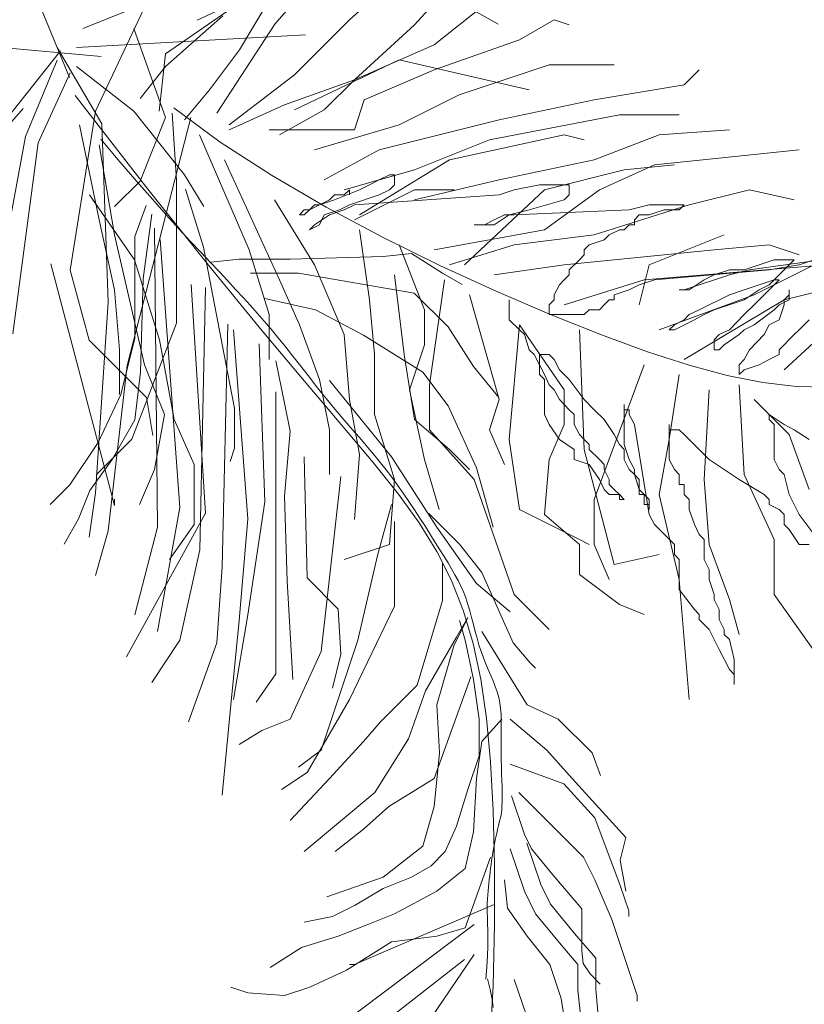
# Model space of a CAD drawing. Units: millimetres. Extents: x 595116 to 630915, y 909473 to 920225.
# Tile 84 of 134: x 629720.161 to 629724.653, y 919270.048 to 919275.684. Entities that reach past the tile are written whole.
import ezdxf

# ---------------------------------------------------------------- set-up
doc = ezdxf.new("R2010")
doc.units = ezdxf.units.MM
doc.layers.add('Dimension', color=3, linetype='Continuous', lineweight=18)
doc.layers.add('L-PLNT', color=85, linetype='Continuous', lineweight=13)
doc.styles.get("Standard").update_dxf_attribs({"font": 'arial.ttf'})
doc.dimstyles.new('ISO-25', dxfattribs={"dimtxt": 9, "dimasz": 6, "dimexe": 1.25, "dimexo": 0.625, "dimtad": 1, "dimlunit": 4, "dimtxsty": 'Standard', "dimcen": 2.5, "dimadec": 0, "dimazin": 0, "dimtfac": 1, "dimtmove": 0, "dimatfit": 3, "dimfxl": 1, "dimarcsym": 0})

# ---------------------------------------------------------------- blocks, each defined once
blk = doc.blocks.new('A$C4FB75ABC')
for p, q in [((2.6324, 2.4053), (2.7073, 2.2214)), ((3.0207, 2.3031), (3.1093, 2.4053)), ((3.1344, 2.3096), (3.2259, 2.3934)), ((3.2335, 2.302), (3.3174, 2.3934)), ((2.7277, 2.2964), (2.8733, 2.3546)), ((2.8539, 2.2576), (2.9801, 2.3449)), ((2.9022, 2.3089), (3.0036, 2.3566)), ((2.8248, 2.3352), (2.7471, 2.1703)), ((2.9666, 2.2638), (3.0123, 2.3401)), ((3.264, 2.2715), (3.3403, 2.3324)), ((3.3079, 2.3327), (3.3615, 2.3029)), ((2.8539, 2.2382), (2.9413, 2.3158)), ((2.9321, 2.167), (3.0207, 2.3031)), ((3.0505, 2.2257), (3.1344, 2.3096)), ((3.142, 2.2181), (3.2335, 2.302)), ((3.3937, 2.2791), (3.447, 2.3096)), ((3.447, 2.3096), (3.4699, 2.302)), ((2.718, 2.2673), (3.0675, 2.2867)), ((2.8054, 2.2964), (2.8539, 2.1606)), ((2.7559, 2.2536), (2.4852, 2.2785)), ((3.142, 2.2181), (3.264, 2.2715)), ((3.264, 2.2334), (3.3937, 2.2791)), ((2.6937, 2.2623), (2.4825, 1.9967)), ((2.6889, 2.2673), (2.7568, 2.1509)), ((2.8442, 2.1703), (2.8539, 2.2576)), ((2.9208, 2.2029), (2.9666, 2.2638)), ((2.6889, 2.2479), (2.6404, 2.1315)), ((2.718, 2.2382), (2.8054, 2.1703)), ((2.8151, 2.1897), (2.8539, 2.2382)), ((3.0505, 2.1724), (3.2106, 2.2486)), ((3.2106, 2.2486), (3.4089, 2.2029)), ((3.3021, 2.1952), (3.4394, 2.241)), ((3.4394, 2.241), (3.5385, 2.241)), ((2.7083, 2.2285), (2.6598, 2.1218)), ((2.9513, 2.1495), (3.0505, 2.2257)), ((3.1572, 2.1876), (3.264, 2.2334)), ((3.6453, 2.2105), (3.6682, 2.2334)), ((3.0352, 2.18), (3.142, 2.2181)), ((3.0962, 2.1724), (3.142, 2.2181)), ((3.508, 2.1876), (3.6453, 2.2105)), ((2.7162, 2.1941), (2.8268, 2.0511)), ((2.8827, 2.1571), (2.9208, 2.2029)), ((3.2106, 2.1495), (3.3021, 2.1952)), ((2.9513, 2.1419), (3.0352, 2.18)), ((3.142, 2.1419), (3.1572, 2.1876)), ((3.3631, 2.1571), (3.508, 2.1876)), ((2.6368, 2.1742), (2.4628, 1.9766)), ((2.7471, 2.1703), (2.7083, 1.9277)), ((2.8054, 2.1703), (2.883, 2.0733)), ((2.864, 2.167), (2.8708, 2.0648)), ((2.9375, 2.1232), (2.8667, 2.1755)), ((3.0276, 2.1343), (3.0962, 2.1724)), ((3.3479, 2.1266), (3.5462, 2.1648)), ((3.5462, 2.1648), (3.6377, 2.1648)), ((2.7225, 2.1495), (2.753, 2.0047)), ((2.7568, 2.1509), (2.7666, 1.8792)), ((2.8927, 2.1606), (2.7957, 1.7822)), ((2.8539, 2.1606), (2.8151, 2.0636)), ((3.081, 2.1114), (3.2106, 2.1495)), ((3.1801, 2.1114), (3.3631, 2.1571)), ((2.9056, 2.1343), (2.9818, 1.9589)), ((3.0123, 2.1419), (3.142, 2.1419)), ((3.2869, 2.0961), (3.4623, 2.1343)), ((3.4623, 2.1343), (3.4928, 2.1266)), ((3.508, 2.0961), (3.6072, 2.1343)), ((3.6072, 2.1343), (3.714, 2.1419)), ((2.6404, 2.1315), (2.5918, 1.8695)), ((2.6598, 2.1218), (2.6209, 1.8307)), ((2.753, 2.119), (2.7759, 1.9818)), ((2.7555, 2.1274), (2.7844, 2.0931)), ((3.0158, 2.0725), (2.9375, 2.1232)), ((3.2335, 2.0809), (3.3479, 2.1266)), ((3.0962, 2.0657), (3.1801, 2.1114)), ((3.5996, 2.0885), (3.8207, 2.1114)), ((2.7844, 2.0931), (2.8104, 2.0628)), ((2.9437, 2.0961), (3.0276, 1.9132)), ((3.1496, 2.0123), (3.2869, 2.0961)), ((3.3631, 2.0657), (3.508, 2.0961)), ((3.5157, 2.0504), (3.5996, 2.0885)), ((3.5538, 2.0809), (3.6301, 2.0885)), ((2.883, 2.0733), (2.9122, 2.0248)), ((3.0992, 2.0238), (3.0158, 2.0725)), ((3.1267, 2.0504), (3.2335, 2.0809)), ((3.1954, 2.0733), (3.1801, 2.0657)), ((3.203, 2.0733), (3.1954, 2.0733)), ((3.203, 2.058), (3.203, 2.0733)), ((3.4318, 2.0504), (3.5538, 2.0809)), ((2.8151, 2.0636), (2.7763, 2.0248)), ((2.8104, 2.0628), (2.8339, 2.0359)), ((2.8708, 2.0648), (2.8708, 1.8469)), ((3.1649, 2.058), (3.1496, 2.0504)), ((3.1801, 2.0657), (3.1649, 2.058)), ((3.1954, 2.0504), (3.203, 2.058)), ((3.2335, 2.0352), (3.3631, 2.0657)), ((3.4242, 2.058), (3.386, 2.0504)), ((3.4699, 2.058), (3.4242, 2.058)), ((3.4699, 2.0428), (3.4699, 2.058)), ((2.7378, 2.0428), (2.8064, 1.9437)), ((2.8268, 2.0511), (2.9214, 1.9326)), ((2.8844, 2.0512), (2.9117, 1.9627)), ((3.1039, 2.0352), (3.1115, 2.0428)), ((3.1496, 2.0504), (3.1115, 2.0352)), ((3.1115, 2.0428), (3.1267, 2.0428)), ((3.1267, 2.0428), (3.1344, 2.0504)), ((3.1344, 2.0504), (3.1344, 2.0428)), ((3.1344, 2.0275), (3.1801, 2.0428)), ((3.142, 2.0047), (3.2335, 2.0504)), ((3.3631, 2.0428), (3.142, 2.0275)), ((3.1801, 2.0428), (3.1954, 2.0504)), ((3.2335, 2.0504), (3.2945, 2.0504)), ((3.3098, 1.9361), (3.4318, 2.0504)), ((3.386, 2.0504), (3.3631, 2.0428)), ((3.4318, 1.9894), (3.5157, 2.0504)), ((3.4623, 2.0352), (3.4699, 2.0428)), ((3.6529, 2.0275), (3.7445, 2.0504)), ((3.7445, 2.0504), (3.8131, 2.0352)), ((2.8339, 2.0359), (2.8551, 2.0121)), ((3.02, 2.0352), (3.081, 1.9361)), ((3.0734, 2.0199), (3.081, 2.0275)), ((3.0886, 2.0275), (3.0734, 2.0199)), ((3.081, 2.0275), (3.0886, 2.0275)), ((3.1115, 2.0352), (3.0886, 2.0275)), ((3.0886, 2.0275), (3.1039, 2.0352)), ((3.1191, 2.0199), (3.1344, 2.0275)), ((3.142, 2.0275), (3.1267, 2.0199)), ((3.4089, 2.0199), (3.4623, 2.0352)), ((3.508, 1.9818), (3.6529, 2.0275)), ((3.5919, 2.0275), (3.5614, 2.0199)), ((3.6453, 2.0275), (3.5919, 2.0275)), ((3.6377, 2.0199), (3.6453, 2.0275)), ((2.8244, 2.0263), (2.8071, 1.979)), ((2.833, 2.0134), (2.8201, 1.9144)), ((3.0581, 2.0123), (3.0657, 2.0199)), ((3.0657, 2.0123), (3.0581, 2.0123)), ((3.0734, 2.0199), (3.0657, 2.0123)), ((3.0657, 2.0199), (3.0734, 2.0199)), ((3.1039, 2.0123), (3.081, 1.9971)), ((3.0886, 1.9971), (3.0962, 2.0123)), ((3.0962, 2.0123), (3.1191, 2.0199)), ((3.1858, 1.9776), (3.0992, 2.0238)), ((3.1267, 2.0199), (3.1039, 2.0123)), ((3.3708, 2.0123), (3.3555, 2.0047)), ((3.3555, 1.9971), (3.3784, 2.0123)), ((3.386, 2.0123), (3.3708, 2.0123)), ((3.3784, 2.0123), (3.4089, 2.0199)), ((3.5614, 2.0199), (3.386, 2.0123)), ((3.5691, 2.0047), (3.5767, 2.0123)), ((3.5767, 2.0123), (3.5919, 2.0123)), ((3.5919, 2.0123), (3.6148, 2.0199)), ((3.6148, 2.0199), (3.6377, 2.0199)), ((2.753, 2.0047), (2.7759, 1.898)), ((2.8551, 2.0121), (2.8744, 1.9909)), ((3.3555, 2.0047), (3.3403, 1.9971)), ((3.5691, 1.9971), (3.5691, 2.0047)), ((2.8373, 1.9919), (2.8416, 1.5357)), ((2.8744, 1.9909), (2.8918, 1.9721)), ((3.081, 1.9971), (3.0734, 1.9894)), ((3.0734, 1.9894), (3.0886, 1.9971)), ((3.1496, 1.9894), (3.1649, 1.8827)), ((3.264, 1.9589), (3.4318, 1.9894)), ((3.3403, 1.9971), (3.325, 1.9971)), ((3.325, 1.9971), (3.3555, 1.9971)), ((3.5309, 1.9818), (3.5462, 1.9894)), ((3.5462, 1.9894), (3.5538, 1.9894)), ((3.5538, 1.9894), (3.5614, 1.9971)), ((3.5614, 1.9971), (3.5691, 1.9971)), ((2.7759, 1.9818), (2.8217, 1.7836)), ((2.8071, 1.979), (2.8071, 1.9015)), ((2.8459, 1.9747), (2.876, 1.5659)), ((2.8918, 1.9721), (2.9078, 1.955)), ((3.2732, 1.9345), (3.1858, 1.9776)), ((3.386, 1.9666), (3.508, 1.9818)), ((3.5004, 1.9666), (3.5233, 1.9742)), ((3.5233, 1.9742), (3.5309, 1.9818)), ((3.5919, 1.9361), (3.7063, 1.9818)), ((2.9078, 1.955), (2.9225, 1.9395)), ((2.9117, 1.9627), (2.9458, 1.7856)), ((2.9818, 1.9589), (3.0123, 1.8599)), ((3.186, 1.9488), (3.2291, 1.9531)), ((3.2106, 1.9666), (3.2488, 1.8675)), ((3.2291, 1.9531), (3.2764, 1.923)), ((3.2869, 1.9361), (3.386, 1.9666)), ((3.4623, 1.9361), (3.6911, 1.9589)), ((3.4928, 1.9589), (3.5004, 1.9666)), ((3.4928, 1.9513), (3.4928, 1.9589)), ((3.6911, 1.9589), (3.775, 1.9666)), ((3.7521, 1.8903), (3.8894, 1.9589)), ((3.775, 1.9666), (3.8207, 1.9513)), ((2.6792, 1.9375), (2.7763, 1.5688)), ((2.8064, 1.9437), (2.8446, 1.8217)), ((2.9225, 1.9395), (2.9361, 1.925)), ((2.9234, 1.9402), (2.9664, 1.9445)), ((2.9664, 1.9445), (3.0439, 1.9445)), ((3.0439, 1.9445), (3.186, 1.9488)), ((3.4699, 1.9285), (3.4852, 1.9437)), ((3.4852, 1.9437), (3.4928, 1.9513)), ((3.7826, 1.9437), (3.7368, 1.9285)), ((3.7445, 1.9285), (3.9122, 1.9513)), ((3.7826, 1.9132), (3.8131, 1.9437)), ((3.8131, 1.9437), (3.7826, 1.9437)), ((3.7978, 1.8827), (4.0495, 1.9437)), ((3.8665, 1.9513), (3.8207, 1.9361)), ((2.7083, 1.9277), (2.7374, 1.821)), ((2.9214, 1.9326), (3.0014, 1.8351)), ((2.9361, 1.925), (2.9489, 1.9114)), ((2.9837, 1.923), (3.0569, 1.923)), ((3.0569, 1.923), (3.2334, 1.8929)), ((3.081, 1.9361), (3.1267, 1.8294)), ((3.3593, 1.8951), (3.2732, 1.9345)), ((3.2764, 1.923), (3.3066, 1.9058)), ((3.3555, 1.9208), (3.4623, 1.9361)), ((3.4699, 1.9208), (3.4699, 1.9285)), ((3.5767, 1.8751), (3.5919, 1.9361)), ((3.5843, 1.9132), (3.8665, 1.9361)), ((3.775, 1.9285), (3.5996, 1.9132)), ((3.714, 1.9285), (3.6911, 1.9208)), ((3.7368, 1.9285), (3.714, 1.9285)), ((3.714, 1.9208), (3.7445, 1.9285)), ((3.8207, 1.9361), (3.775, 1.9285)), ((2.8201, 1.9144), (2.8158, 1.7724)), ((2.9489, 1.9114), (2.9609, 1.8985)), ((3.0276, 1.9132), (3.0581, 1.8446)), ((3.203, 1.9208), (3.2182, 1.7989)), ((3.2793, 1.9132), (3.2564, 1.7531)), ((3.4547, 1.9056), (3.4623, 1.9132)), ((3.4623, 1.9132), (3.4699, 1.9208)), ((3.4623, 1.8751), (3.5843, 1.9132)), ((3.5996, 1.9132), (3.5767, 1.9056)), ((3.6453, 1.898), (3.714, 1.9208)), ((3.6758, 1.9132), (3.6529, 1.898)), ((3.6911, 1.9208), (3.6758, 1.9132)), ((3.7368, 1.898), (3.7826, 1.9132)), ((3.7826, 1.9132), (3.775, 1.9056)), ((3.7826, 1.9056), (3.7902, 1.9132)), ((3.7902, 1.9132), (3.7826, 1.9132)), ((2.7759, 1.898), (2.7836, 1.8065)), ((2.8071, 1.9015), (2.8071, 1.8241)), ((2.8933, 1.9058), (2.9148, 1.5573)), ((2.9148, 1.9015), (2.9062, 1.5013)), ((2.9609, 1.8985), (2.9724, 1.8861)), ((3.2334, 1.8929), (3.285, 1.8413)), ((3.4421, 1.8597), (3.3593, 1.8951)), ((3.447, 1.8903), (3.4547, 1.9056)), ((3.5614, 1.898), (3.5385, 1.8903)), ((3.5767, 1.9056), (3.5614, 1.898)), ((3.6529, 1.898), (3.6377, 1.898)), ((3.6377, 1.898), (3.6453, 1.898)), ((3.714, 1.8903), (3.7368, 1.898)), ((3.7597, 1.898), (3.7368, 1.8827)), ((3.7597, 1.8827), (3.7826, 1.9056)), ((3.775, 1.9056), (3.7597, 1.898)), ((3.8055, 1.8903), (3.8055, 1.898)), ((3.8055, 1.898), (3.8055, 1.8827)), ((2.7666, 1.8792), (2.7471, 1.5882)), ((2.9724, 1.8861), (2.9834, 1.874)), ((3.0052, 1.8843), (3.0827, 1.8671)), ((3.1649, 1.8827), (3.1725, 1.7989)), ((3.3174, 1.8903), (3.3631, 1.7303)), ((3.3784, 1.8827), (3.3784, 1.8522)), ((3.4394, 1.8751), (3.447, 1.8827)), ((3.447, 1.8827), (3.447, 1.8903)), ((3.5309, 1.8827), (3.5233, 1.8751)), ((3.5385, 1.8827), (3.5309, 1.8827)), ((3.5385, 1.8903), (3.5385, 1.8827)), ((3.6072, 1.837), (3.7521, 1.8903)), ((3.6453, 1.7913), (3.7978, 1.8827)), ((3.6682, 1.8675), (3.714, 1.8903)), ((3.7368, 1.8827), (3.6911, 1.8675)), ((3.7521, 1.8751), (3.7597, 1.8827)), ((3.8055, 1.8827), (3.7902, 1.8751)), ((3.7978, 1.8827), (3.8055, 1.8903)), ((3.7978, 1.8751), (3.7978, 1.8827)), ((2.9834, 1.874), (2.994, 1.862)), ((3.0827, 1.8671), (3.1559, 1.8284)), ((3.2488, 1.8675), (3.2488, 1.8141)), ((3.4394, 1.8599), (3.4394, 1.8751)), ((3.5004, 1.8675), (3.4928, 1.8599)), ((3.5157, 1.8675), (3.5004, 1.8675)), ((3.5233, 1.8751), (3.5157, 1.8675)), ((3.6529, 1.8599), (3.6682, 1.8675)), ((3.6911, 1.8675), (3.6758, 1.8599)), ((3.7368, 1.8599), (3.7521, 1.8751)), ((3.7826, 1.8675), (3.7521, 1.8446)), ((3.7902, 1.8751), (3.7826, 1.8675)), ((3.7902, 1.8522), (3.7978, 1.8751)), ((3.7978, 1.776), (3.897, 1.8675)), ((2.994, 1.862), (3.0045, 1.8499)), ((3.0045, 1.8499), (3.0149, 1.8377)), ((3.0123, 1.8599), (3.0123, 1.7913)), ((3.3784, 1.8522), (3.3937, 1.837)), ((3.4928, 1.8599), (3.4394, 1.8599)), ((3.5192, 1.829), (3.4421, 1.8597)), ((3.6606, 1.8522), (3.6301, 1.837)), ((3.6301, 1.8446), (3.6453, 1.8522)), ((3.6453, 1.8522), (3.6529, 1.8599)), ((3.6758, 1.8599), (3.6606, 1.8522)), ((3.714, 1.837), (3.7368, 1.8599)), ((3.775, 1.8446), (3.7902, 1.8522)), ((3.836, 1.8522), (3.8207, 1.837)), ((2.8708, 1.8469), (2.8027, 1.6699)), ((2.9492, 1.8456), (2.9406, 1.4755)), ((2.9578, 1.837), (2.9794, 1.5486)), ((3.0014, 1.8351), (3.0686, 1.7552)), ((3.0149, 1.8377), (3.0253, 1.8251)), ((3.0581, 1.8446), (3.0886, 1.7608)), ((3.285, 1.8413), (3.3238, 1.781)), ((3.3937, 1.8446), (3.3784, 1.6693)), ((3.3937, 1.8446), (3.4623, 1.7455)), ((3.3937, 1.837), (3.4013, 1.8294)), ((3.4852, 1.837), (3.4928, 1.6541)), ((3.6224, 1.837), (3.6301, 1.8446)), ((3.6301, 1.837), (3.6224, 1.837)), ((3.6987, 1.8294), (3.714, 1.837)), ((3.7368, 1.837), (3.7292, 1.8294)), ((3.7521, 1.8446), (3.7368, 1.837)), ((3.7673, 1.8294), (3.775, 1.8446)), ((3.8207, 1.837), (3.8131, 1.8294)), ((2.7374, 1.821), (2.8248, 1.7337)), ((2.8071, 1.8241), (2.7856, 1.738)), ((2.8446, 1.8217), (2.8674, 1.6998)), ((3.0253, 1.8251), (3.0358, 1.8122)), ((3.1267, 1.8294), (3.1344, 1.7303)), ((3.1559, 1.8284), (3.2463, 1.7724)), ((3.4013, 1.8294), (3.4089, 1.8065)), ((3.5892, 1.8034), (3.5192, 1.829)), ((3.6911, 1.8217), (3.6987, 1.8294)), ((3.6911, 1.8065), (3.6911, 1.8217)), ((3.7292, 1.8294), (3.7063, 1.8141)), ((3.7445, 1.8065), (3.7673, 1.8294)), ((3.8131, 1.8294), (3.7902, 1.8065)), ((2.7836, 1.8065), (2.7836, 1.7379)), ((2.9966, 1.8154), (3.0052, 1.5745)), ((3.0358, 1.8122), (3.0461, 1.7993)), ((3.2488, 1.8141), (3.2259, 1.7455)), ((3.4089, 1.8065), (3.4165, 1.7989)), ((3.6527, 1.7828), (3.5892, 1.8034)), ((3.6987, 1.8065), (3.6911, 1.8065)), ((3.7063, 1.8141), (3.6987, 1.8065)), ((3.7368, 1.7913), (3.7445, 1.8065)), ((3.7902, 1.8065), (3.7902, 1.7989)), ((3.0224, 1.7896), (3.0353, 1.7251)), ((3.0461, 1.7993), (3.0562, 1.7866)), ((3.1725, 1.7989), (3.1725, 1.7074)), ((3.2182, 1.7989), (3.2335, 1.6998)), ((3.4165, 1.7989), (3.4242, 1.7836)), ((3.4242, 1.7684), (3.4242, 1.7989)), ((3.4242, 1.7989), (3.4394, 1.7989)), ((3.4394, 1.7989), (3.447, 1.7913)), ((3.447, 1.7913), (3.4547, 1.776)), ((3.7292, 1.7836), (3.7368, 1.7913)), ((3.775, 1.7913), (3.7597, 1.7836)), ((3.7902, 1.7989), (3.775, 1.7913)), ((2.7957, 1.7822), (2.7666, 1.53)), ((2.8158, 1.7724), (2.8071, 1.6993)), ((2.8217, 1.7836), (2.8522, 1.7074)), ((2.9458, 1.7856), (2.9594, 1.7175)), ((3.0562, 1.7866), (3.0659, 1.7741)), ((3.0659, 1.7741), (3.0752, 1.7623)), ((3.2463, 1.7724), (3.285, 1.7208)), ((3.3238, 1.781), (3.3625, 1.7337)), ((3.4242, 1.7836), (3.4318, 1.7684)), ((3.4547, 1.776), (3.4699, 1.7608)), ((3.5843, 1.7836), (3.508, 1.5778)), ((3.7109, 1.7672), (3.6527, 1.7828)), ((3.7292, 1.7684), (3.7292, 1.7836)), ((3.7368, 1.776), (3.7292, 1.7684)), ((3.7597, 1.7836), (3.7368, 1.776)), ((3.0752, 1.7623), (3.084, 1.7511)), ((3.0886, 1.7608), (3.1039, 1.6845)), ((3.1042, 1.7595), (3.1989, 1.6433)), ((3.4318, 1.7608), (3.4242, 1.7684)), ((3.4318, 1.7684), (3.4394, 1.7531)), ((3.4318, 1.7074), (3.4318, 1.7608)), ((3.4699, 1.7608), (3.4928, 1.7303)), ((3.6377, 1.7684), (3.6224, 1.6693)), ((3.7651, 1.7564), (3.7109, 1.7672)), ((3.0224, 1.7423), (3.0224, 1.312)), ((3.0686, 1.7552), (3.1246, 1.6894)), ((3.084, 1.7511), (3.0921, 1.7408)), ((3.2259, 1.7455), (3.2488, 1.6388)), ((3.2564, 1.7531), (3.2564, 1.6845)), ((3.4394, 1.7531), (3.447, 1.7455)), ((3.447, 1.7455), (3.4547, 1.7303)), ((3.4623, 1.7455), (3.4623, 1.6922)), ((3.6834, 1.7455), (3.6758, 1.6083)), ((3.7292, 1.7531), (3.7368, 1.6159)), ((3.8165, 1.7504), (3.7651, 1.7564)), ((3.8664, 1.749), (3.8165, 1.7504)), ((2.7856, 1.738), (2.7512, 1.6648)), ((2.8248, 1.7337), (2.8345, 1.6755)), ((3.0921, 1.7408), (3.0994, 1.7316)), ((3.0994, 1.7316), (3.1062, 1.7232)), ((3.1344, 1.7303), (3.1496, 1.6464)), ((3.3631, 1.7303), (3.3479, 1.6845)), ((3.4547, 1.7303), (3.4699, 1.715)), ((3.4928, 1.7303), (3.508, 1.715)), ((3.7521, 1.7303), (3.8055, 1.6769)), ((2.9594, 1.7175), (2.9594, 1.6563)), ((3.0353, 1.7251), (3.0439, 1.682)), ((3.1062, 1.7232), (3.1126, 1.7155)), ((3.1126, 1.7155), (3.1186, 1.7083)), ((3.285, 1.7208), (3.3281, 1.6261)), ((3.4699, 1.715), (3.4775, 1.7074)), ((3.508, 1.715), (3.5233, 1.6998)), ((3.5538, 1.7227), (3.5538, 1.715)), ((3.5538, 1.6617), (3.5538, 1.7227)), ((3.5538, 1.715), (3.5614, 1.715)), ((3.5614, 1.715), (3.5614, 1.7074)), ((2.8071, 1.6993), (2.7727, 1.639)), ((2.8522, 1.7074), (2.8369, 1.6236)), ((2.8674, 1.6998), (2.8979, 1.6312)), ((3.1186, 1.7083), (3.1246, 1.7013)), ((3.1246, 1.7013), (3.1305, 1.6944)), ((3.1725, 1.7074), (3.203, 1.6083)), ((3.2335, 1.6998), (3.2869, 1.6541)), ((3.4394, 1.6922), (3.4318, 1.7074)), ((3.4775, 1.7074), (3.4775, 1.6922)), ((3.5233, 1.6998), (3.5385, 1.6769)), ((3.5614, 1.7074), (3.5691, 1.6922)), ((3.775, 1.6998), (3.775, 1.7074)), ((3.775, 1.7074), (3.7978, 1.6922)), ((3.7826, 1.6922), (3.775, 1.6998)), ((3.0439, 1.682), (3.0353, 1.5831)), ((3.1039, 1.6845), (3.1039, 1.6159)), ((3.1246, 1.6894), (3.1709, 1.6342)), ((3.1305, 1.6944), (3.1367, 1.6873)), ((3.1367, 1.6873), (3.1432, 1.6798)), ((3.2564, 1.6845), (3.325, 1.6083)), ((3.3479, 1.6845), (3.3708, 1.6312)), ((3.4547, 1.6693), (3.4394, 1.6922)), ((3.4623, 1.6922), (3.4394, 1.6388)), ((3.4775, 1.6922), (3.4852, 1.6769)), ((3.5691, 1.6922), (3.5919, 1.555)), ((3.6224, 1.6922), (3.6224, 1.6845)), ((3.6224, 1.6388), (3.6224, 1.6922)), ((3.6224, 1.6845), (3.6377, 1.6845)), ((3.6377, 1.6845), (3.6453, 1.6769)), ((3.7826, 1.6388), (3.7826, 1.6922)), ((3.7978, 1.6922), (3.8131, 1.6845)), ((3.8131, 1.6845), (3.836, 1.6693)), ((2.8027, 1.6699), (2.7482, 1.6154)), ((3.1432, 1.6798), (3.1502, 1.6718)), ((3.1502, 1.6718), (3.1576, 1.6632)), ((3.3784, 1.6693), (3.3937, 1.5626)), ((3.4775, 1.6541), (3.4547, 1.6693)), ((3.4852, 1.6769), (3.4928, 1.6693)), ((3.4928, 1.6693), (3.5004, 1.6617)), ((3.5385, 1.6769), (3.5462, 1.6617)), ((3.6224, 1.6693), (3.6072, 1.5855)), ((3.6453, 1.6769), (3.6682, 1.6541)), ((3.8055, 1.6769), (3.836, 1.5931)), ((2.7512, 1.6648), (2.7081, 1.6003)), ((2.9594, 1.6563), (2.9526, 1.6358)), ((3.1576, 1.6632), (3.1654, 1.654)), ((3.1654, 1.654), (3.1735, 1.6443)), ((3.2869, 1.6541), (3.3174, 1.6236)), ((3.4775, 1.6388), (3.4775, 1.6541)), ((3.4928, 1.6541), (3.5385, 1.4787)), ((3.5004, 1.6617), (3.5004, 1.6541)), ((3.5004, 1.6541), (3.5157, 1.6388)), ((3.5462, 1.6617), (3.5538, 1.6541)), ((3.5614, 1.6388), (3.5538, 1.6617)), ((3.5538, 1.6541), (3.5538, 1.6388)), ((3.6682, 1.6541), (3.6834, 1.6388)), ((2.7727, 1.639), (2.7383, 1.5917)), ((3.0655, 1.6433), (3.0698, 1.4583)), ((3.1496, 1.6464), (3.142, 1.5473)), ((3.1735, 1.6443), (3.1819, 1.634)), ((3.1989, 1.6433), (3.2678, 1.5357)), ((3.2488, 1.6388), (3.2716, 1.5626)), ((3.4394, 1.6388), (3.4318, 1.555)), ((3.5004, 1.6312), (3.4775, 1.6388)), ((3.5157, 1.6388), (3.5233, 1.6312)), ((3.5538, 1.6388), (3.5614, 1.6236)), ((3.5691, 1.6236), (3.5614, 1.6388)), ((3.6301, 1.6236), (3.6224, 1.6388)), ((3.6834, 1.6388), (3.7292, 1.6083)), ((3.7902, 1.6236), (3.7826, 1.6388)), ((2.8369, 1.6236), (2.8141, 1.5702)), ((2.8979, 1.6312), (2.8979, 1.5397)), ((3.1709, 1.6342), (3.2091, 1.5863)), ((3.1819, 1.634), (3.1904, 1.6232)), ((3.1904, 1.6232), (3.1991, 1.6119)), ((3.3281, 1.6261), (3.3539, 1.5357)), ((3.5157, 1.6083), (3.5004, 1.6312)), ((3.5233, 1.6312), (3.5233, 1.6236)), ((3.5233, 1.6236), (3.5309, 1.6083)), ((3.5614, 1.6236), (3.5691, 1.6159)), ((3.5691, 1.6159), (3.5691, 1.6236)), ((3.6377, 1.6159), (3.6301, 1.6236)), ((3.7978, 1.6159), (3.7902, 1.6236)), ((3.1214, 1.6132), (3.1042, 1.4583)), ((3.203, 1.6083), (3.1954, 1.5092)), ((3.1991, 1.6119), (3.2078, 1.6)), ((3.325, 1.6083), (3.386, 1.433)), ((3.5233, 1.5931), (3.5157, 1.6083)), ((3.5309, 1.6083), (3.5309, 1.6007)), ((3.5691, 1.6159), (3.5767, 1.6083)), ((3.5767, 1.5931), (3.5691, 1.6159)), ((3.5767, 1.6083), (3.5767, 1.5855)), ((3.6377, 1.6007), (3.6377, 1.6159)), ((3.6758, 1.6083), (3.6834, 1.5092)), ((3.7292, 1.6083), (3.7673, 1.5855)), ((3.7368, 1.6159), (3.7826, 1.5168)), ((3.8055, 1.5855), (3.7978, 1.6159)), ((2.7081, 1.6003), (2.678, 1.5702)), ((3.2078, 1.6), (3.2166, 1.5877)), ((3.5309, 1.5855), (3.5233, 1.5931)), ((3.5309, 1.6007), (3.5385, 1.5931)), ((3.5385, 1.5931), (3.5462, 1.5855)), ((3.5843, 1.5855), (3.5767, 1.5931)), ((3.6453, 1.6007), (3.6377, 1.6007)), ((3.6453, 1.5855), (3.6453, 1.6007)), ((2.7383, 1.5917), (2.721, 1.5486)), ((2.7471, 1.5882), (2.7374, 1.5203)), ((2.7763, 1.5688), (2.7763, 1.5785)), ((3.0353, 1.5831), (3.0396, 1.454)), ((3.2091, 1.5863), (3.241, 1.5422)), ((3.2166, 1.5877), (3.2252, 1.575)), ((3.508, 1.5778), (3.508, 1.5092)), ((3.5462, 1.5855), (3.5309, 1.5855)), ((3.5462, 1.5855), (3.5462, 1.5778)), ((3.5538, 1.5778), (3.5462, 1.5855)), ((3.5462, 1.5778), (3.5538, 1.5778)), ((3.5767, 1.5855), (3.5843, 1.5855)), ((3.5843, 1.5855), (3.5843, 1.5702)), ((3.5919, 1.5778), (3.5843, 1.5855)), ((3.5919, 1.5626), (3.5919, 1.5778)), ((3.6072, 1.5855), (3.6377, 1.4559)), ((3.6529, 1.5778), (3.6453, 1.5855)), ((3.6529, 1.5626), (3.6529, 1.5778)), ((3.7673, 1.5855), (3.775, 1.5778)), ((3.775, 1.5778), (3.775, 1.5702)), ((3.8131, 1.5702), (3.8055, 1.5855)), ((2.876, 1.5659), (2.8416, 1.3765)), ((3.0052, 1.5745), (2.9794, 1.4023)), ((3.1989, 1.5702), (3.1774, 1.4927)), ((3.2252, 1.575), (3.2338, 1.5622)), ((3.2338, 1.5622), (3.2421, 1.5493)), ((3.3937, 1.5626), (3.4852, 1.5168)), ((3.5843, 1.5702), (3.5919, 1.5702)), ((3.5919, 1.5702), (3.5919, 1.5626)), ((3.6606, 1.5397), (3.6529, 1.5626)), ((3.775, 1.5702), (3.7902, 1.5626)), ((3.7902, 1.5626), (3.7978, 1.555)), ((3.8207, 1.555), (3.8131, 1.5702)), ((2.721, 1.5486), (2.6995, 1.5099)), ((2.9148, 1.5573), (2.7942, 1.3378)), ((2.9794, 1.5486), (2.9664, 1.3937)), ((3.2421, 1.5493), (3.2503, 1.5367)), ((3.2549, 1.5573), (3.3023, 1.5099)), ((3.4318, 1.555), (3.4852, 1.5092)), ((3.5919, 1.555), (3.5996, 1.5397)), ((3.7978, 1.555), (3.7978, 1.5397)), ((3.8436, 1.5245), (3.8207, 1.555)), ((2.8416, 1.5357), (2.8071, 1.4023)), ((2.8979, 1.5397), (2.8598, 1.4864)), ((3.2032, 1.5443), (3.2032, 1.4152)), ((3.241, 1.5422), (3.2678, 1.4987)), ((3.2503, 1.5367), (3.258, 1.5243)), ((3.2678, 1.5357), (3.3281, 1.4497)), ((3.5996, 1.5397), (3.6301, 1.5092)), ((3.6682, 1.5245), (3.6606, 1.5397)), ((3.7978, 1.5397), (3.8055, 1.5321)), ((3.8055, 1.5321), (3.8207, 1.5092)), ((2.7666, 1.53), (2.7471, 1.462)), ((3.258, 1.5243), (3.2655, 1.5125)), ((3.4852, 1.5168), (3.5004, 1.5092)), ((3.6758, 1.5168), (3.6682, 1.5245)), ((3.6758, 1.4864), (3.6758, 1.5168)), ((3.7826, 1.5168), (3.7826, 1.433)), ((3.1954, 1.5092), (3.1267, 1.4864)), ((3.2655, 1.5125), (3.2724, 1.5013)), ((3.3023, 1.5099), (3.3367, 1.4669)), ((3.4852, 1.5092), (3.4852, 1.4635)), ((3.508, 1.5092), (3.5309, 1.4559)), ((3.6301, 1.5092), (3.6301, 1.494)), ((3.6834, 1.5092), (3.714, 1.4254)), ((3.8207, 1.5092), (3.836, 1.5092)), ((2.9062, 1.5013), (2.876, 1.3636)), ((3.1774, 1.4927), (3.1473, 1.3636)), ((3.2678, 1.4987), (3.2902, 1.4543)), ((3.2724, 1.5013), (3.2789, 1.491)), ((3.2789, 1.491), (3.2849, 1.4813)), ((3.5385, 1.4787), (3.6072, 1.494)), ((3.6301, 1.494), (3.6377, 1.4864)), ((2.9406, 1.4755), (2.932, 1.3593)), ((3.2764, 1.4798), (3.2764, 1.4239)), ((3.2849, 1.4813), (3.2904, 1.4721)), ((3.2904, 1.4721), (3.2955, 1.4632)), ((3.6377, 1.4864), (3.6377, 1.4406)), ((3.6834, 1.4711), (3.6758, 1.4864)), ((3.0698, 1.4583), (3.1171, 1.4109)), ((3.1042, 1.4583), (3.0913, 1.3464)), ((3.2955, 1.4632), (3.3002, 1.4545)), ((3.3367, 1.4669), (3.3841, 1.3593)), ((3.4852, 1.4635), (3.5462, 1.4178)), ((3.6834, 1.4559), (3.6834, 1.4711)), ((3.0396, 1.454), (3.0483, 1.3034)), ((3.2902, 1.4543), (3.3086, 1.4079)), ((3.3002, 1.4545), (3.3045, 1.4458)), ((3.3045, 1.4458), (3.3084, 1.437)), ((3.3281, 1.4497), (3.3798, 1.4066)), ((3.6377, 1.4559), (3.6529, 1.2729)), ((3.6911, 1.433), (3.6834, 1.4559)), ((3.3084, 1.437), (3.3119, 1.4278)), ((3.3119, 1.4278), (3.3151, 1.4181)), ((3.386, 1.433), (3.4394, 1.3796)), ((3.6377, 1.4406), (3.6606, 1.4101)), ((3.6911, 1.4254), (3.6911, 1.433)), ((3.7826, 1.433), (3.8741, 1.3034)), ((3.2032, 1.4152), (3.1344, 1.2732)), ((3.2764, 1.4239), (3.2377, 1.2948)), ((3.3151, 1.4181), (3.3181, 1.4081)), ((3.5462, 1.4178), (3.5843, 1.4025)), ((3.6987, 1.4101), (3.6911, 1.4254)), ((3.714, 1.4254), (3.7292, 1.372)), ((2.9794, 1.4023), (2.9578, 1.2732)), ((3.1171, 1.4109), (3.1214, 1.3421)), ((3.2937, 1.355), (3.3152, 1.398)), ((3.298, 1.3679), (3.3152, 1.398)), ((3.3086, 1.4079), (3.3233, 1.3583)), ((3.3181, 1.4081), (3.3209, 1.3978)), ((3.3209, 1.3978), (3.3236, 1.3873)), ((3.6606, 1.4101), (3.6682, 1.4025)), ((3.6682, 1.4025), (3.6682, 1.3949)), ((3.6987, 1.3949), (3.6987, 1.4101)), ((2.9664, 1.3937), (2.9535, 1.2646)), ((3.3023, 1.3937), (3.3109, 1.3636)), ((3.3236, 1.3873), (3.3263, 1.3768)), ((3.6682, 1.3949), (3.6834, 1.3796)), ((3.7063, 1.3796), (3.6987, 1.3949)), ((3.2506, 1.2861), (3.298, 1.3679)), ((3.3263, 1.3768), (3.3291, 1.3664)), ((3.3367, 1.3765), (3.4056, 1.2646)), ((3.6834, 1.3796), (3.6987, 1.3492)), ((3.7063, 1.372), (3.7063, 1.3796)), ((3.714, 1.3644), (3.7063, 1.372)), ((2.876, 1.3636), (2.833, 1.2991)), ((2.932, 1.3593), (2.889, 1.2388)), ((3.1473, 1.3636), (3.0913, 1.1958)), ((3.2678, 1.2646), (3.2937, 1.355)), ((3.3109, 1.3636), (3.3238, 1.3034)), ((3.3233, 1.3583), (3.3348, 1.3042)), ((3.3291, 1.3664), (3.332, 1.3561)), ((3.332, 1.3561), (3.3352, 1.3462)), ((3.3841, 1.3593), (3.4099, 1.3292)), ((3.7216, 1.3339), (3.714, 1.3644)), ((3.0913, 1.3464), (3.0439, 1.2431)), ((3.1214, 1.3421), (3.1085, 1.2905)), ((3.3352, 1.3462), (3.3388, 1.3366)), ((3.3388, 1.3366), (3.3425, 1.3274)), ((3.6987, 1.3492), (3.714, 1.3187)), ((3.3425, 1.3274), (3.3463, 1.3185)), ((3.4099, 1.3292), (3.4185, 1.3206)), ((3.7216, 1.2958), (3.7216, 1.3339)), ((3.0224, 1.312), (2.9923, 1.2689)), ((3.3195, 1.3077), (3.2635, 1.1527)), ((3.3463, 1.3185), (3.3501, 1.3098)), ((3.3501, 1.3098), (3.3537, 1.3013)), ((3.714, 1.3187), (3.7216, 1.311)), ((3.7216, 1.311), (3.7216, 1.2958)), ((3.2377, 1.2948), (3.1817, 1.2388)), ((3.3238, 1.3034), (3.3324, 1.2431)), ((3.3348, 1.3042), (3.3434, 1.2446)), ((3.3537, 1.3013), (3.357, 1.2929)), ((3.357, 1.2929), (3.3598, 1.2846)), ((3.2248, 1.213), (3.2506, 1.2861)), ((3.3598, 1.2846), (3.3622, 1.2762)), ((2.9535, 1.2646), (2.9406, 1.1269)), ((3.1344, 1.2732), (3.0698, 1.1614)), ((3.2721, 1.1915), (3.2678, 1.2646)), ((3.3622, 1.2762), (3.3639, 1.2677)), ((3.3639, 1.2677), (3.365, 1.2592)), ((3.4056, 1.2646), (3.453, 1.2431)), ((3.365, 1.2592), (3.3657, 1.2504)), ((3.3657, 1.2504), (3.366, 1.2415)), ((3.0439, 1.2431), (3.0009, 1.2259)), ((3.1817, 1.2388), (3.1559, 1.2087)), ((3.3324, 1.2431), (3.3324, 1.1872)), ((3.3367, 1.2087), (3.3669, 1.2431)), ((3.3434, 1.2446), (3.3495, 1.1781)), ((3.366, 1.2415), (3.366, 1.2322)), ((3.366, 1.2322), (3.366, 1.2227)), ((3.3798, 1.2431), (3.4357, 1.1958)), ((3.453, 1.2431), (3.5046, 1.1915)), ((3.0009, 1.2259), (2.9664, 1.2044)), ((3.366, 1.2227), (3.3658, 1.2129)), ((3.1559, 1.2087), (3.1042, 1.1527)), ((3.1731, 1.1312), (3.2248, 1.213)), ((3.3281, 1.1527), (3.3367, 1.2087)), ((3.3658, 1.2129), (3.3658, 1.2027)), ((3.3658, 1.2027), (3.3658, 1.1921)), ((3.0913, 1.1958), (3.0569, 1.17)), ((3.2635, 1.1097), (3.2721, 1.1915)), ((3.3324, 1.1872), (3.3152, 1.1355)), ((3.3658, 1.1921), (3.366, 1.1812)), ((3.4357, 1.1958), (3.4745, 1.1527)), ((3.5046, 1.1915), (3.5175, 1.1571)), ((3.3495, 1.1781), (3.3535, 1.1037)), ((3.366, 1.1812), (3.3663, 1.1704)), ((3.3798, 1.1743), (3.4616, 1.1441)), ((3.0698, 1.1614), (3.031, 1.1355)), ((3.3663, 1.1704), (3.3667, 1.1597)), ((3.3667, 1.1597), (3.367, 1.1494)), ((3.1042, 1.1527), (3.0439, 1.0882)), ((3.2635, 1.1527), (3.1946, 1.1097)), ((3.3238, 1.071), (3.3281, 1.1527)), ((3.367, 1.1494), (3.3673, 1.1397)), ((3.4616, 1.1441), (3.5089, 1.0925)), ((3.4745, 1.1527), (3.5563, 1.0624)), ((3.0655, 1.0409), (3.1731, 1.1312)), ((3.3152, 1.1355), (3.298, 1.0796)), ((3.3673, 1.1397), (3.3675, 1.1308)), ((3.3675, 1.1308), (3.3676, 1.1228)), ((3.3927, 1.1312), (3.44, 1.0839)), ((3.3675, 1.116), (3.3672, 1.1101)), ((3.3676, 1.1228), (3.3675, 1.116)), ((3.3816, 1.1261), (3.4013, 1.0669)), ((3.1946, 1.1097), (3.1559, 1.0753)), ((3.2463, 1.0495), (3.2635, 1.1097)), ((3.3535, 1.1037), (3.3557, 1.0207)), ((3.3657, 1.0966), (3.3649, 1.0928)), ((3.3663, 1.1006), (3.3657, 1.0966)), ((3.3668, 1.1051), (3.3663, 1.1006)), ((3.3672, 1.1101), (3.3668, 1.1051)), ((3.3631, 1.0852), (3.362, 1.081)), ((3.364, 1.0891), (3.3631, 1.0852)), ((3.3649, 1.0928), (3.364, 1.0891)), ((3.44, 1.0839), (3.4917, 1.0323)), ((3.5089, 1.0925), (3.5477, 0.9892)), ((3.1559, 1.0753), (3.1128, 1.0409)), ((3.298, 1.0796), (3.2807, 1.0409)), ((3.3109, 1.015), (3.3238, 1.071)), ((3.3586, 1.0667), (3.3574, 1.0614)), ((3.3598, 1.0717), (3.3586, 1.0667)), ((3.3609, 1.0765), (3.3598, 1.0717)), ((3.362, 1.081), (3.3609, 1.0765)), ((3.4013, 1.0669), (3.4121, 1.0454)), ((3.3563, 1.056), (3.3551, 1.0505)), ((3.3574, 1.0614), (3.3563, 1.056)), ((3.4053, 1.0537), (3.4263, 0.991)), ((3.5563, 1.0624), (3.5477, 1.028)), ((3.186, 1.0021), (3.2463, 1.0495)), ((3.2807, 1.0409), (3.2592, 1.0193)), ((3.3531, 1.039), (3.3522, 1.0332)), ((3.3541, 1.0448), (3.3531, 1.039)), ((3.3551, 1.0505), (3.3541, 1.0448)), ((3.3798, 1.0452), (3.4013, 0.9806)), ((3.4121, 1.0454), (3.4447, 1.0056)), ((3.3496, 1.0323), (3.3109, 0.9247)), ((3.3506, 1.0215), (3.3499, 1.0156)), ((3.3514, 1.0274), (3.3506, 1.0215)), ((3.3522, 1.0332), (3.3514, 1.0274)), ((3.4917, 1.0323), (3.5089, 0.9978)), ((3.5477, 1.028), (3.5563, 0.9806)), ((3.2592, 1.0193), (3.2291, 1.0021)), ((3.2678, 0.9806), (3.3109, 1.015)), ((3.3492, 1.0097), (3.3485, 1.0039)), ((3.3499, 1.0156), (3.3492, 1.0097)), ((3.3557, 1.0207), (3.3558, 0.9307)), ((3.0999, 0.972), (3.186, 1.0021)), ((3.2291, 1.0021), (3.186, 0.9849)), ((3.3471, 0.9925), (3.3465, 0.9868)), ((3.3478, 0.9982), (3.3471, 0.9925)), ((3.3485, 1.0039), (3.3478, 0.9982)), ((3.3712, 0.9978), (3.3755, 0.9548)), ((3.4447, 1.0056), (3.4889, 0.9539)), ((3.5089, 0.9978), (3.5348, 0.9376)), ((3.186, 0.9849), (3.143, 0.9591)), ((3.2032, 0.9462), (3.2678, 0.9806)), ((3.3459, 0.981), (3.3454, 0.9751)), ((3.3465, 0.9868), (3.3459, 0.981)), ((3.4013, 0.9806), (3.4185, 0.9462)), ((3.4263, 0.991), (3.4413, 0.9609)), ((3.5477, 0.9892), (3.5606, 0.9505)), ((3.3447, 0.9623), (3.3446, 0.9554)), ((3.345, 0.9689), (3.3447, 0.9623)), ((3.3454, 0.9751), (3.345, 0.9689)), ((3.143, 0.9591), (3.1085, 0.9419)), ((3.3555, 0.9604), (3.142, 0.8689)), ((3.1602, 0.929), (3.2032, 0.9462)), ((3.3446, 0.9554), (3.3447, 0.9479)), ((3.3447, 0.9479), (3.3449, 0.9399)), ((3.3755, 0.9548), (3.4056, 0.9118)), ((3.4185, 0.9462), (3.4573, 0.8989)), ((3.4413, 0.9609), (3.4779, 0.9162)), ((3.4889, 0.9539), (3.4889, 0.8899)), ((3.5606, 0.9505), (3.5606, 0.9419)), ((3.1085, 0.9419), (3.0655, 0.9333)), ((3.3449, 0.9399), (3.3453, 0.931)), ((3.5348, 0.9376), (3.5735, 0.8214)), ((3.325, 0.9299), (3.0505, 0.7241)), ((3.1171, 0.9118), (3.1602, 0.929)), ((3.3109, 0.9247), (3.2678, 0.9118)), ((3.3453, 0.931), (3.3456, 0.921)), ((3.3456, 0.921), (3.3457, 0.9097)), ((3.3558, 0.9307), (3.3535, 0.836)), ((3.4779, 0.9162), (3.5101, 0.8787)), ((3.0612, 0.8946), (3.1171, 0.9118)), ((3.1989, 0.9032), (3.1301, 0.8601)), ((3.2678, 0.9118), (3.1989, 0.9032)), ((3.3457, 0.9097), (3.3456, 0.8969)), ((3.4056, 0.9118), (3.44, 0.8687)), ((3.0138, 0.8644), (3.0612, 0.8946)), ((3.3456, 0.8969), (3.3451, 0.8822)), ((3.4573, 0.8989), (3.4831, 0.8687)), ((3.4889, 0.8899), (3.4909, 0.8704)), ((3.3098, 0.8766), (3.1344, 0.7394)), ((3.325, 0.8842), (3.1954, 0.6936)), ((3.3451, 0.8822), (3.3441, 0.8655)), ((3.5101, 0.8787), (3.5101, 0.8314)), ((3.1301, 0.8601), (3.0741, 0.8343)), ((3.142, 0.8689), (3.1344, 0.8689)), ((3.3441, 0.8655), (3.3424, 0.8466)), ((3.44, 0.8687), (3.4573, 0.8171)), ((3.4831, 0.8687), (3.4831, 0.83)), ((3.4909, 0.8704), (3.5015, 0.8546)), ((3.3453, 0.8472), (3.3494, 0.8306)), ((3.386, 0.8461), (3.508, 0.4878)), ((3.5015, 0.8546), (3.5172, 0.8388)), ((2.9794, 0.8257), (2.9535, 0.8343)), ((3.0741, 0.8343), (3.0353, 0.8214)), ((3.3535, 0.836), (3.3484, 0.7387)), ((3.3494, 0.8306), (3.3521, 0.8161)), ((3.4831, 0.83), (3.4874, 0.787)), ((3.5101, 0.8314), (3.5136, 0.7963)), ((3.0353, 0.8214), (2.9794, 0.8257)), ((3.3521, 0.8161), (3.3535, 0.8034)), ((3.4573, 0.8171), (3.4659, 0.7655)), ((3.5735, 0.8214), (3.5735, 0.8128))]:
    blk.add_line(p, q)
blk = doc.blocks.new('*D216')
at = {"layer": 'Defpoints', "color": 0, "transparency": 16777216}
for p in [(629743.5408, 919411.9276), (629505.0408, 919411.8279), (629743.5408, 918832.3776)]:
    blk.add_point(p, dxfattribs=at)
at = {"layer": 'Dimension', "color": 0, "lineweight": -2, "transparency": 16777216}
for p, q in [((629743.5408, 919411.3026), (629743.5408, 918831.1276)), ((629505.0408, 919411.2029), (629505.0408, 918831.1276)), ((629511.0408, 918832.3776), (629737.5408, 918832.3776))]:
    blk.add_line(p, q, dxfattribs=at)
at = {"layer": 'Dimension', "color": 0, "transparency": 16777216}
for points in [[(629511.0408, 918833.3776), (629511.0408, 918831.3776), (629505.0408, 918832.3776)], [(629737.5408, 918833.3776), (629737.5408, 918831.3776), (629743.5408, 918832.3776)]]:
    blk.add_solid(points, dxfattribs=at)
at = {"layer": 'Dimension', "color": 0, "transparency": 16777216, "insert": (629624.2908, 918837.656), "char_height": 9, "attachment_point": 5}
blk.add_mtext('19\'-10 1/2"', dxfattribs=at)

msp = doc.modelspace()

# ---------------------------------------------------------------- block references
at = {"layer": 'L-PLNT', "xscale": 3.753413438031968, "yscale": 3.753413438031968, "zscale": 3.753413438031968}
msp.add_blockref('A$C4FB75ABC', (629710.2837, 919267.0144), dxfattribs=at)

# ---------------------------------------------------------------- dimensions: what is measured, and where the dimension line sits
at = {"layer": 'Dimension'}
dim = msp.add_linear_dim(base=(629743.5408, 918832.3776), p1=(629505.0408, 919411.8279), p2=(629743.5408, 919411.9276), dimstyle='ISO-25', override={"dimdec": 1, "dimlfac": 1, "dimrnd": 0, "dimzin": 1, "dimdsep": 46, "dimlunit": 4, "dimfrac": 2}, dxfattribs=at)
dim.commit()
dim.dimension.update_dxf_attribs({"geometry": '*D216', "text_midpoint": (629624.2908, 918837.656)})

doc.saveas('drawing.dxf')
